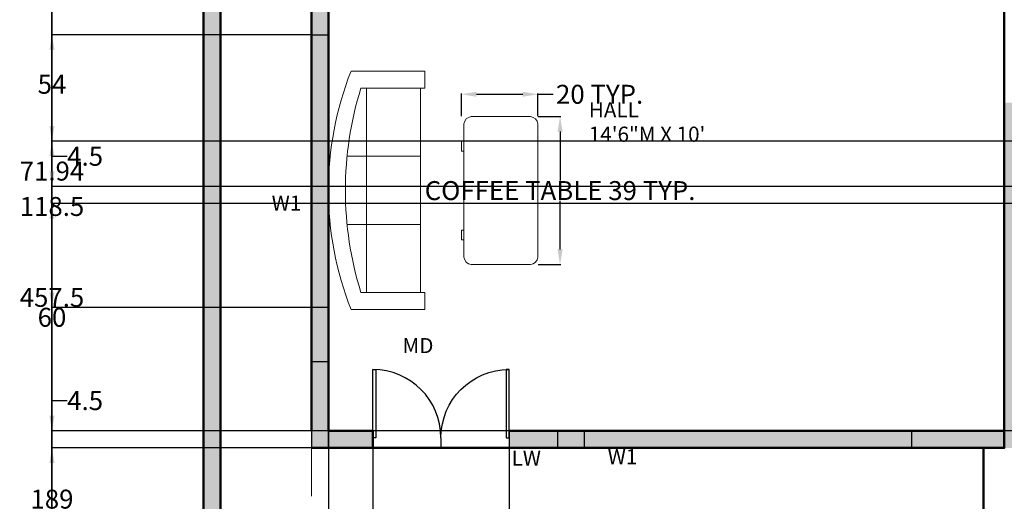
# Model space of a CAD drawing. Units: inches. Extents: x -12 to 887, y 330 to 874.
# Tile 2 of 9: x -7 to 253, y 548 to 675. Entities that reach past the tile are written whole.
import ezdxf

# ---------------------------------------------------------------- set-up
doc = ezdxf.new("R2010")
doc.units = ezdxf.units.IN
doc.header["$MEASUREMENT"] = 0
doc.linetypes.add('DASHED', pattern=[19.05, 12.7, -6.35])
for name, color, linetype, lineweight in [('A-ANNO-DIMS', 2, 'Continuous', 18), ('A-ANNO-TEXT', 3, 'Continuous', 18), ('A-AREA-IDEN', 7, 'Continuous', 18), ('A-DOOR', 4, 'Continuous', 25), ('A-FURN', 9, 'Continuous', 18), ('A-GLAZ', 4, 'Continuous', 25), ('A-WALL', 7, 'Continuous', 50), ('A-WALL-OVHD', 8, 'DASHED', 18), ('A-WALL-PATT', 5, 'Continuous', 13)]:
    doc.layers.add(name, color=color, linetype=linetype, lineweight=lineweight)
doc.styles.get("Standard").update_dxf_attribs({"font": 'arial.ttf'})
doc.dimstyles.get("Standard").update_dxf_attribs({"dimtxt": 5, "dimasz": 4, "dimexe": 0.18, "dimexo": 0.0625, "dimgap": 0.09, "dimtad": 0, "dimtih": 1, "dimtoh": 1, "dimdec": 1, "dimzin": 0, "dimdsep": 46, "dimlunit": 4, "dimtxsty": 'Standard', "dimcen": 0.09, "dimadec": 0, "dimazin": 0, "dimtfac": 1, "dimtdec": 1, "dimtofl": 0, "dimtmove": 0, "dimatfit": 3, "dimfxl": 1, "dimtolj": 1, "dimtzin": 0, "dimarcsym": 0})

# ---------------------------------------------------------------- blocks, each defined once
blk = doc.blocks.new('*U5')
for p, q in [((0, 0), (0, -6)), ((40, 0), (40, -6))]:
    blk.add_line(p, q)
blk.add_lwpolyline([(0, 0), (0, 40), (1.75, 40), (1.75, 0)], close=True)
blk.add_arc((0, 0), 40, 0, 90)
blk = doc.blocks.new('Sofa - Roundback 7 ft.')
for p, q in [((-12.00002, -32.4421), (-12.00003, -6.5971)), ((11.99997, -32.4421), (11.99998, -6.5971)), ((-36.000027, -34), (-36.000027, -11.4696)), ((-35.999844, -13.3819), (35.9998, -13.3819)), ((35.99998, -34), (35.99998, -11.4696)), ((-36.000027, -32.4421), (35.99998, -32.4421))]:
    blk.add_line(p, q)
for points in [[(-36.000027, -34), (-42.000027, -34), (-42.000027, -8)], [(41.99998, -8), (41.99998, -34), (35.99998, -34)]]:
    blk.add_lwpolyline(points)
for centre, radius, start, end in [((0, -114.25), 114.25, 68.43141, 111.5686), ((-0.00001, -127.1968), 121.1968, 72.72033, 107.2797)]:
    blk.add_arc(centre, radius, start, end)
blk = doc.blocks.new('Desk - 30 x 60 in.')
for p, q in [((-26.999995, 0), (26.999995, 0)), ((-29.999995, -27), (-29.999995, -3)), ((29.999995, -3), (29.999995, -27)), ((26.999995, -30), (-26.999995, -30)), ((-20.000005, -30), (-20.000005, -31)), ((-20.000005, -31), (-16.000005, -31)), ((-16.000005, -31), (-16.000005, -30)), ((15.999995, -31), (15.999995, -30)), ((19.999995, -31), (15.999995, -31)), ((19.999995, -30), (19.999995, -31))]:
    blk.add_line(p, q)
for centre, start, end in [((-26.499995, -3.5), 98.1301, 171.8699), ((26.499995, -3.5), 8.130102, 81.8699), ((-26.499995, -26.5), 188.1301, 261.8699), ((26.499995, -26.5), 278.1301, 351.8699)]:
    blk.add_arc(centre, 3.535534, start, end)
blk = doc.blocks.new('*D34')
at = {"layer": 'A-ANNO-DIMS', "color": 0, "lineweight": -2, "transparency": 16777216}
for p, q in [((130.31, 649.66), (136.29, 649.66)), ((136.11, 645.66), (136.11, 632.78)), ((136.11, 614.55), (136.11, 627.42)), ((130.31, 610.55), (136.29, 610.55))]:
    blk.add_line(p, q, dxfattribs=at)
at = {"layer": 'A-ANNO-DIMS', "color": 0, "transparency": 16777216}
for points in [[(135.45, 645.66), (136.78, 645.66), (136.11, 649.66)], [(135.45, 614.55), (136.78, 614.55), (136.11, 610.55)]]:
    blk.add_solid(points, dxfattribs=at)
at = {"layer": 'Defpoints', "color": 0, "transparency": 16777216}
for p in [(130.25, 649.66), (130.25, 610.55), (136.11, 610.55)]:
    blk.add_point(p, dxfattribs=at)
at = {"layer": 'A-ANNO-DIMS', "color": 0, "transparency": 16777216, "insert": (136.11, 630.1), "char_height": 5, "attachment_point": 5}
blk.add_mtext('\\A1;COFFEE TABLE 39 TYP.', dxfattribs=at)
blk = doc.blocks.new('*D35')
at = {"layer": 'A-ANNO-DIMS', "color": 0, "lineweight": -2, "transparency": 16777216}
for p, q in [((110.04, 649.72), (110.04, 655.7)), ((114.04, 655.52), (126.25, 655.52)), ((130.25, 649.72), (130.25, 655.7)), ((130.25, 655.52), (134.25, 655.52))]:
    blk.add_line(p, q, dxfattribs=at)
at = {"layer": 'A-ANNO-DIMS', "color": 0, "transparency": 16777216}
for points in [[(114.04, 656.19), (114.04, 654.86), (110.04, 655.52)], [(126.25, 656.19), (126.25, 654.86), (130.25, 655.52)]]:
    blk.add_solid(points, dxfattribs=at)
at = {"layer": 'Defpoints', "color": 0, "transparency": 16777216}
for p in [(130.25, 655.52), (110.04, 649.66), (130.25, 649.66)]:
    blk.add_point(p, dxfattribs=at)
at = {"layer": 'A-ANNO-DIMS', "color": 0, "transparency": 16777216, "insert": (146.55, 655.52), "char_height": 5, "attachment_point": 5}
blk.add_mtext('\\A1;20 TYP.', dxfattribs=at)
blk = doc.blocks.new('*D53')
at = {"layer": 'A-ANNO-DIMS', "color": 0, "lineweight": -2, "transparency": 16777216}
for p, q in [((41.86, 830.66), (1.75, 830.66)), ((1.93, 826.66), (1.93, 604.54)), ((1.93, 377.16), (1.93, 599.28)), ((41.86, 373.16), (1.75, 373.16))]:
    blk.add_line(p, q, dxfattribs=at)
at = {"layer": 'A-ANNO-DIMS', "color": 0, "transparency": 16777216}
for points in [[(1.26, 826.66), (2.59, 826.66), (1.93, 830.66)], [(1.26, 377.16), (2.59, 377.16), (1.93, 373.16)]]:
    blk.add_solid(points, dxfattribs=at)
at = {"layer": 'Defpoints', "color": 0, "transparency": 16777216}
for p in [(1.93, 830.66), (41.93, 830.66), (41.93, 373.16)]:
    blk.add_point(p, dxfattribs=at)
at = {"layer": 'A-ANNO-DIMS', "color": 0, "transparency": 16777216, "insert": (1.93, 601.91), "char_height": 5, "attachment_point": 5}
blk.add_mtext('\\A1;457.5', dxfattribs=at)
blk = doc.blocks.new('*D55')
at = {"layer": 'A-ANNO-DIMS', "color": 0, "lineweight": -2, "transparency": 16777216}
for p, q in [((70.36, 562.16), (1.75, 562.16)), ((1.93, 558.16), (1.93, 474.8)), ((1.93, 386.16), (1.93, 469.52)), ((70.36, 382.16), (1.75, 382.16))]:
    blk.add_line(p, q, dxfattribs=at)
at = {"layer": 'A-ANNO-DIMS', "color": 0, "transparency": 16777216}
for points in [[(1.26, 558.16), (2.59, 558.16), (1.93, 562.16)], [(1.26, 386.16), (2.59, 386.16), (1.93, 382.16)]]:
    blk.add_solid(points, dxfattribs=at)
at = {"layer": 'Defpoints', "color": 0, "transparency": 16777216}
for p in [(1.93, 562.16), (70.43, 562.16), (70.43, 382.16)]:
    blk.add_point(p, dxfattribs=at)
at = {"layer": 'A-ANNO-DIMS', "color": 0, "transparency": 16777216, "insert": (1.93, 472.16), "char_height": 5, "attachment_point": 5}
blk.add_mtext('\\A1;180', dxfattribs=at)
blk = doc.blocks.new('*D56')
at = {"layer": 'A-ANNO-DIMS', "color": 0, "lineweight": -2, "transparency": 16777216}
for p, q in [((1.93, 570.66), (1.93, 574.66)), ((1.93, 574.66), (5.93, 574.66)), ((74.86, 566.66), (1.75, 566.66)), ((70.36, 562.16), (1.75, 562.16)), ((1.93, 558.16), (1.93, 554.16))]:
    blk.add_line(p, q, dxfattribs=at)
at = {"layer": 'A-ANNO-DIMS', "color": 0, "transparency": 16777216}
for points in [[(1.26, 570.66), (2.59, 570.66), (1.93, 566.66)], [(1.26, 558.16), (2.59, 558.16), (1.93, 562.16)]]:
    blk.add_solid(points, dxfattribs=at)
at = {"layer": 'Defpoints', "color": 0, "transparency": 16777216}
for p in [(1.93, 566.66), (74.93, 566.66), (70.43, 562.16)]:
    blk.add_point(p, dxfattribs=at)
at = {"layer": 'A-ANNO-DIMS', "color": 0, "transparency": 16777216, "insert": (10.69, 574.66), "char_height": 5, "attachment_point": 5}
blk.add_mtext('\\A1;4.5', dxfattribs=at)
blk = doc.blocks.new('*D57')
at = {"layer": 'A-ANNO-DIMS', "color": 0, "lineweight": -2, "transparency": 16777216}
for p, q in [((74.86, 685.16), (1.75, 685.16)), ((1.93, 681.16), (1.93, 628.55)), ((1.93, 570.66), (1.93, 623.27)), ((74.86, 566.66), (1.75, 566.66))]:
    blk.add_line(p, q, dxfattribs=at)
at = {"layer": 'A-ANNO-DIMS', "color": 0, "transparency": 16777216}
for points in [[(1.26, 681.16), (2.59, 681.16), (1.93, 685.16)], [(1.26, 570.66), (2.59, 570.66), (1.93, 566.66)]]:
    blk.add_solid(points, dxfattribs=at)
at = {"layer": 'Defpoints', "color": 0, "transparency": 16777216}
for p in [(1.93, 685.16), (74.93, 685.16), (74.93, 566.66)]:
    blk.add_point(p, dxfattribs=at)
at = {"layer": 'A-ANNO-DIMS', "color": 0, "transparency": 16777216, "insert": (1.93, 625.91), "char_height": 5, "attachment_point": 5}
blk.add_mtext('\\A1;118.5', dxfattribs=at)
blk = doc.blocks.new('*D67')
at = {"layer": 'A-ANNO-DIMS', "color": 0, "lineweight": -2, "transparency": 16777216}
for p, q in [((319.86, 626.66), (1.75, 626.66)), ((1.93, 622.66), (1.93, 599.3)), ((1.93, 570.66), (1.93, 594.02)), ((319.86, 566.66), (1.75, 566.66))]:
    blk.add_line(p, q, dxfattribs=at)
at = {"layer": 'A-ANNO-DIMS', "color": 0, "transparency": 16777216}
for points in [[(1.26, 622.66), (2.59, 622.66), (1.93, 626.66)], [(1.26, 570.66), (2.59, 570.66), (1.93, 566.66)]]:
    blk.add_solid(points, dxfattribs=at)
at = {"layer": 'Defpoints', "color": 0, "transparency": 16777216}
for p in [(1.93, 626.66), (319.93, 626.66), (319.93, 566.66)]:
    blk.add_point(p, dxfattribs=at)
at = {"layer": 'A-ANNO-DIMS', "color": 0, "transparency": 16777216, "insert": (1.93, 596.66), "char_height": 5, "attachment_point": 5}
blk.add_mtext('\\A1;60', dxfattribs=at)
blk = doc.blocks.new('*D68')
at = {"layer": 'A-ANNO-DIMS', "color": 0, "lineweight": -2, "transparency": 16777216}
for p, q in [((1.93, 635.16), (1.93, 639.16)), ((1.93, 639.16), (5.93, 639.16)), ((319.86, 631.16), (1.75, 631.16)), ((319.86, 626.66), (1.75, 626.66)), ((1.93, 622.66), (1.93, 618.66))]:
    blk.add_line(p, q, dxfattribs=at)
at = {"layer": 'A-ANNO-DIMS', "color": 0, "transparency": 16777216}
for points in [[(1.26, 635.16), (2.59, 635.16), (1.93, 631.16)], [(1.26, 622.66), (2.59, 622.66), (1.93, 626.66)]]:
    blk.add_solid(points, dxfattribs=at)
at = {"layer": 'Defpoints', "color": 0, "transparency": 16777216}
for p in [(1.93, 631.16), (319.93, 631.16), (319.93, 626.66)]:
    blk.add_point(p, dxfattribs=at)
at = {"layer": 'A-ANNO-DIMS', "color": 0, "transparency": 16777216, "insert": (10.69, 639.16), "char_height": 5, "attachment_point": 5}
blk.add_mtext('\\A1;4.5', dxfattribs=at)
blk = doc.blocks.new('*D69')
at = {"layer": 'A-ANNO-DIMS', "color": 0, "lineweight": -2, "transparency": 16777216}
for p, q in [((319.86, 685.16), (1.75, 685.16)), ((1.93, 681.16), (1.93, 660.79)), ((1.93, 635.16), (1.93, 655.53)), ((319.86, 631.16), (1.75, 631.16))]:
    blk.add_line(p, q, dxfattribs=at)
at = {"layer": 'A-ANNO-DIMS', "color": 0, "transparency": 16777216}
for points in [[(1.26, 681.16), (2.59, 681.16), (1.93, 685.16)], [(1.26, 635.16), (2.59, 635.16), (1.93, 631.16)]]:
    blk.add_solid(points, dxfattribs=at)
at = {"layer": 'Defpoints', "color": 0, "transparency": 16777216}
for p in [(1.93, 685.16), (319.93, 685.16), (319.93, 631.16)]:
    blk.add_point(p, dxfattribs=at)
at = {"layer": 'A-ANNO-DIMS', "color": 0, "transparency": 16777216, "insert": (1.93, 658.16), "char_height": 5, "attachment_point": 5}
blk.add_mtext('\\A1;54', dxfattribs=at)
blk = doc.blocks.new('*D76')
at = {"layer": 'A-ANNO-DIMS', "color": 0, "lineweight": -2, "transparency": 16777216}
for p, q in [((74.93, 566.6), (74.93, 332.98)), ((86.65, 566.6), (86.65, 332.98)), ((78.93, 333.16), (82.65, 333.16)), ((86.65, 333.16), (90.65, 333.16))]:
    blk.add_line(p, q, dxfattribs=at)
at = {"layer": 'A-ANNO-DIMS', "color": 0, "transparency": 16777216}
for points in [[(78.93, 333.83), (78.93, 332.49), (74.93, 333.16)], [(82.65, 333.83), (82.65, 332.49), (86.65, 333.16)]]:
    blk.add_solid(points, dxfattribs=at)
at = {"layer": 'Defpoints', "color": 0, "transparency": 16777216}
for p in [(74.93, 566.66), (86.65, 566.66), (86.65, 333.16)]:
    blk.add_point(p, dxfattribs=at)
at = {"layer": 'A-ANNO-DIMS', "color": 0, "transparency": 16777216, "insert": (98.91, 333.16), "char_height": 5, "attachment_point": 5}
blk.add_mtext('\\A1;11.72', dxfattribs=at)
blk = doc.blocks.new('*D77')
at = {"layer": 'A-ANNO-DIMS', "color": 0, "lineweight": -2, "transparency": 16777216}
for p, q in [((86.65, 566.6), (86.65, 332.98)), ((122.7, 566.6), (122.7, 332.98)), ((90.65, 333.16), (96.13, 333.16)), ((118.7, 333.16), (113.22, 333.16))]:
    blk.add_line(p, q, dxfattribs=at)
at = {"layer": 'A-ANNO-DIMS', "color": 0, "transparency": 16777216}
for points in [[(90.65, 333.83), (90.65, 332.49), (86.65, 333.16)], [(118.7, 333.83), (118.7, 332.49), (122.7, 333.16)]]:
    blk.add_solid(points, dxfattribs=at)
at = {"layer": 'Defpoints', "color": 0, "transparency": 16777216}
for p in [(86.65, 566.66), (122.7, 566.66), (122.7, 333.16)]:
    blk.add_point(p, dxfattribs=at)
at = {"layer": 'A-ANNO-DIMS', "color": 0, "transparency": 16777216, "insert": (104.67, 333.16), "char_height": 5, "attachment_point": 5}
blk.add_mtext('\\A1;36.05', dxfattribs=at)
blk = doc.blocks.new('*D82')
at = {"layer": 'A-ANNO-DIMS', "color": 0, "lineweight": -2, "transparency": 16777216}
for p, q in [((70.36, 671.22), (1.75, 671.22)), ((1.93, 667.22), (1.93, 637.89)), ((1.93, 603.27), (1.93, 632.6)), ((70.36, 599.27), (1.75, 599.27))]:
    blk.add_line(p, q, dxfattribs=at)
at = {"layer": 'A-ANNO-DIMS', "color": 0, "transparency": 16777216}
for points in [[(1.26, 667.22), (2.59, 667.22), (1.93, 671.22)], [(1.26, 603.27), (2.59, 603.27), (1.93, 599.27)]]:
    blk.add_solid(points, dxfattribs=at)
at = {"layer": 'Defpoints', "color": 0, "transparency": 16777216}
for p in [(70.43, 671.22), (1.93, 599.27), (70.43, 599.27)]:
    blk.add_point(p, dxfattribs=at)
at = {"layer": 'A-ANNO-DIMS', "color": 0, "transparency": 16777216, "insert": (1.93, 635.24), "char_height": 5, "attachment_point": 5}
blk.add_mtext('\\A1;71.94', dxfattribs=at)
blk = doc.blocks.new('*D101')
at = {"layer": 'A-ANNO-DIMS', "color": 0, "lineweight": -2, "transparency": 16777216}
for p, q in [((493.01, 643.16), (1.75, 643.16)), ((1.93, 639.16), (1.93, 551.3)), ((1.93, 458.16), (1.93, 546.02)), ((493.01, 454.16), (1.75, 454.16))]:
    blk.add_line(p, q, dxfattribs=at)
at = {"layer": 'A-ANNO-DIMS', "color": 0, "transparency": 16777216}
for points in [[(1.26, 639.16), (2.59, 639.16), (1.93, 643.16)], [(1.26, 458.16), (2.59, 458.16), (1.93, 454.16)]]:
    blk.add_solid(points, dxfattribs=at)
at = {"layer": 'Defpoints', "color": 0, "transparency": 16777216}
for p in [(1.93, 643.16), (493.07, 643.16), (493.07, 454.16)]:
    blk.add_point(p, dxfattribs=at)
at = {"layer": 'A-ANNO-DIMS', "color": 0, "transparency": 16777216, "insert": (1.93, 548.66), "char_height": 5, "attachment_point": 5}
blk.add_mtext('\\A1;189', dxfattribs=at)
blk = doc.blocks.new('*D102')
at = {"layer": 'A-ANNO-DIMS', "color": 0, "lineweight": -2, "transparency": 16777216}
for p, q in [((493.01, 821.66), (1.75, 821.66)), ((1.93, 817.66), (1.93, 735.05)), ((1.93, 647.16), (1.93, 729.77)), ((493.01, 643.16), (1.75, 643.16))]:
    blk.add_line(p, q, dxfattribs=at)
at = {"layer": 'A-ANNO-DIMS', "color": 0, "transparency": 16777216}
for points in [[(1.26, 817.66), (2.59, 817.66), (1.93, 821.66)], [(1.26, 647.16), (2.59, 647.16), (1.93, 643.16)]]:
    blk.add_solid(points, dxfattribs=at)
at = {"layer": 'Defpoints', "color": 0, "transparency": 16777216}
for p in [(1.93, 821.66), (493.07, 821.66), (493.07, 643.16)]:
    blk.add_point(p, dxfattribs=at)
at = {"layer": 'A-ANNO-DIMS', "color": 0, "transparency": 16777216, "insert": (1.93, 732.41), "char_height": 5, "attachment_point": 5}
blk.add_mtext('\\A1;178.5', dxfattribs=at)

msp = doc.modelspace()

# ---------------------------------------------------------------- hatches: boundary and pattern name
at = {"layer": 'A-WALL-PATT'}
h = msp.add_hatch(color=256, dxfattribs=at)
h.dxf.hatch_style = 1
h.paths.add_polyline_path([(253.4263, 830.6611), (94.575, 830.6611), (94.575, 821.6611), (198.9263, 821.6611), (198.9263, 783.3094), (203.4263, 783.3094), (203.4263, 821.6611), (253.4263, 821.6611)], flags=17)
h.paths.add_polyline_path([(415.4263, 830.6611), (392.9263, 830.6611), (392.9263, 821.6611), (410.9263, 821.6611), (410.9263, 701.6611), (410.9263, 382.1611), (392.9263, 382.1611), (392.9263, 450.1611), (383.9263, 450.1611), (383.9263, 382.1611), (253.4263, 382.1611), (46.4263, 382.1611), (46.4263, 821.6611), (67.3199, 821.6611), (67.3199, 830.6611), (41.9263, 830.6611), (41.9263, 373.1611), (253.4263, 373.1611), (415.4263, 373.1611)])
h.paths.add_polyline_path([(364.023, 830.6611), (288.8031, 830.6611), (288.8031, 821.6611), (364.023, 821.6611)], flags=17)
h.paths.add_polyline_path([(257.9263, 821.6611), (253.4263, 821.6611), (253.4263, 749.6611), (203.4263, 749.6611), (203.4263, 759.3094), (198.9263, 759.3094), (198.9263, 745.1611), (253.4263, 745.1611), (253.4263, 735.8547), (257.9263, 735.8547)], flags=17)
h.paths.add_polyline_path([(257.9263, 653.338), (257.0311, 653.338), (253.4263, 653.338), (253.4263, 579.1607), (257.9263, 579.1607)], flags=17)
h.paths.add_polyline_path([(323.9263, 685.1611), (328.2749, 685.1611), (328.2749, 689.6611), (257.9263, 689.6611), (257.9263, 685.1611), (319.9263, 685.1611), (319.9263, 631.1611), (257.9263, 631.1611), (257.9263, 626.6611), (319.9263, 626.6611), (319.9263, 566.6611), (286.6409, 566.6611, -0.00931598), (286.6576, 565.7658), (286.6576, 562.1611), (383.9263, 562.1611), (383.9263, 566.6611), (323.9263, 566.6611)], flags=17)
h.paths.add_polyline_path([(142.5107, 566.6611), (135.5357, 566.6611), (135.5357, 562.1611), (142.5107, 562.1611)], flags=17)
h.paths.add_polyline_path([(253.4263, 566.6611), (229.0035, 566.6611), (229.0035, 562.1611), (253.4263, 562.1611)], flags=17)
h.paths.add_polyline_path([(262.6261, 566.6611), (257.9263, 566.6611), (257.9263, 562.1611), (262.6261, 562.1611)], flags=17)
h.paths.add_polyline_path([(392.9263, 553.5254), (383.9263, 553.5254), (383.9263, 454.1611), (392.9263, 454.1611)], flags=17)
h.paths.add_polyline_path([(353.8031, 418.1611), (247.9263, 418.1611), (247.9263, 414.1611), (353.8031, 414.1611)], flags=17)
h.paths.add_polyline_path([(374.959, 454.1611), (272.0195, 454.1611), (272.0195, 450.1611), (374.959, 450.1611)], flags=17)
h.paths.add_polyline_path([(254.2006, 454.1611), (247.9263, 454.1611), (247.9263, 450.1611), (254.2006, 450.1611)], flags=17)
h = msp.add_hatch(color=256, dxfattribs=at)
h.dxf.hatch_style = 1
h.paths.add_polyline_path([(94.575, 830.6611), (67.3199, 830.6611), (67.3199, 821.6611), (70.4263, 821.6611), (79.4263, 821.6611), (94.575, 821.6611)])
h.paths.add_polyline_path([(288.8031, 830.6611), (257.9263, 830.6611), (253.4263, 830.6611), (253.4263, 821.6611), (288.8031, 821.6611)])
h.paths.add_polyline_path([(74.9263, 696.9265), (70.4263, 696.9265), (70.4263, 678.4656), (74.9263, 678.4656)])
h.paths.add_polyline_path([(74.9263, 584.8756), (70.4263, 584.8756), (70.4263, 562.1611), (74.9263, 562.1611)])
h.paths.add_polyline_path([(135.5357, 566.6611), (122.6994, 566.6611), (122.6994, 562.1611), (135.5357, 562.1611)])
h.paths.add_polyline_path([(257.9263, 579.1607), (253.4263, 579.1607), (253.4263, 562.1611), (257.9263, 562.1611)])
h.paths.add_polyline_path([(272.0195, 454.1611), (254.2006, 454.1611), (254.2006, 450.1611), (272.0195, 450.1611)])
h.paths.add_polyline_path([(392.9263, 454.1611), (374.959, 454.1611), (374.959, 450.1611), (383.9263, 450.1611), (392.9263, 450.1611)])
h.paths.add_polyline_path([(493.0683, 466.4171), (488.5683, 466.4171), (488.5683, 450.1611), (493.0683, 450.1611)])
h.paths.add_polyline_path([(568.6302, 454.1611), (555.938, 454.1611), (555.938, 450.1611), (568.6302, 450.1611)])
h.paths.add_polyline_path([(493.0683, 594.9471), (488.5683, 594.9471), (488.5683, 569.5862), (493.0683, 569.5862)])
h.paths.add_polyline_path([(690.1615, 454.1611), (672.3426, 454.1611), (672.3426, 450.1611), (690.1615, 450.1611)])
h.paths.add_polyline_path([(811.0683, 454.1611), (793.101, 454.1611), (793.101, 450.1611), (802.0683, 450.1611), (811.0683, 450.1611)])
h.paths.add_polyline_path([(811.0683, 578.3606), (802.0683, 578.3606), (802.0683, 566.6611), (802.0683, 553.5254), (811.0683, 553.5254)])
h.paths.add_polyline_path([(811.0683, 701.6611), (802.0683, 701.6611), (802.0683, 689.9616), (802.0683, 676.8259), (811.0683, 676.8259)])
h.paths.add_polyline_path([(811.0683, 830.6611), (782.165, 830.6611), (782.165, 821.6611), (802.0683, 821.6611), (811.0683, 821.6611)])
h.paths.add_polyline_path([(706.9451, 830.6611), (671.5683, 830.6611), (671.5683, 821.6611), (706.9451, 821.6611)])
h.paths.add_polyline_path([(512.717, 830.6611), (485.4619, 830.6611), (485.4619, 821.6611), (488.5683, 821.6611), (512.717, 821.6611)])
h.paths.add_polyline_path([(392.9263, 697.8668), (383.9263, 697.8668), (383.9263, 689.6611), (383.9263, 676.5034), (392.9263, 676.5034)])
h.paths.add_polyline_path([(392.9263, 830.6611), (364.023, 830.6611), (364.023, 821.7357), (392.9263, 821.7357)])
h.paths.add_polyline_path([(392.9263, 619.0434), (383.9263, 619.0434), (383.9263, 588.7499), (392.9263, 588.7499)])
h.paths.add_polyline_path([(392.9263, 578.3606), (383.9263, 578.3606), (383.9263, 566.6611), (383.9263, 553.5254), (392.9263, 553.5254)])
h.paths.add_polyline_path([(257.9263, 699.8547), (253.4263, 699.8547), (253.4263, 697.1611), (253.4263, 677.338), (257.9263, 677.338)])
h.paths.add_polyline_path([(493.0683, 714.3785), (488.5683, 714.3785), (488.5683, 689.6611), (493.0683, 689.6611)])
h.paths.add_polyline_path([(74.9263, 491.4191), (70.4263, 491.4191), (70.4263, 480.7097), (74.9263, 480.7097)])
h = msp.add_hatch(color=256, dxfattribs=at)
h.dxf.hatch_style = 1
h.paths.add_polyline_path([(86.6469, 566.6611), (74.9263, 566.6611), (74.9263, 562.1611), (86.6469, 562.1611)])
h.paths.add_polyline_path([(74.9263, 599.271), (70.4263, 599.271), (70.4263, 584.8756), (74.9263, 584.8756)])
h.paths.add_polyline_path([(74.9263, 678.4656), (70.4263, 678.4656), (70.4263, 671.2153), (74.9263, 671.2153)])
h.paths.add_polyline_path([(74.9263, 709.2627), (70.4263, 709.2627), (70.4263, 696.9265), (74.9263, 696.9265)])
h.paths.add_polyline_path([(74.9263, 821.6611), (70.4263, 821.6611), (70.4263, 749.8953), (74.9263, 749.8953)])
h.paths.add_polyline_path([(383.9263, 689.6611), (352.3064, 689.6611), (352.3064, 686.0564, -0.00931598), (352.2897, 685.1611), (383.9263, 685.1611)])
h.paths.add_polyline_path([(392.9263, 706.6608), (383.9263, 706.6608), (383.9263, 701.6611), (383.9263, 697.8668), (392.9263, 697.8668)])
h.paths.add_polyline_path([(392.9263, 821.7357), (383.9263, 821.7357), (383.9263, 751.0224), (383.9263, 742.7561), (392.9263, 742.7561)])
h.paths.add_polyline_path([(392.9263, 676.5034), (383.9263, 676.5034), (383.9263, 619.0434), (392.9263, 619.0434)])
h.paths.add_polyline_path([(392.9263, 588.7499), (383.9263, 588.7499), (383.9263, 578.3606), (392.9263, 578.3606)])
h = msp.add_hatch(color=256, dxfattribs=at)
h.dxf.hatch_style = 1
h.paths.add_polyline_path([(74.9263, 749.8953), (70.4263, 749.8953), (70.4263, 709.2627), (74.9263, 709.2627)])
h.paths.add_polyline_path([(74.9263, 671.2153), (70.4263, 671.2153), (70.4263, 599.271), (74.9263, 599.271)])
h.paths.add_polyline_path([(229.0035, 566.6611), (142.5107, 566.6611), (142.5107, 562.1611), (229.0035, 562.1611)])
h.paths.add_polyline_path([(392.9263, 742.7561), (383.9263, 742.7561), (383.9263, 706.6608), (392.9263, 706.6608)])
h.paths.add_polyline_path([(656.7304, 454.1611), (582.6585, 454.1611), (582.6585, 450.1611), (656.7304, 450.1611)])
h.paths.add_polyline_path([(493.0683, 557.2595), (488.5683, 557.2595), (488.5683, 492.3446), (493.0683, 492.3446)])
h.paths.add_polyline_path([(493.0683, 781.3634), (488.5683, 781.3634), (488.5683, 728.8273), (493.0683, 728.8273)])
h.paths.add_polyline_path([(811.0683, 756.0738), (802.0683, 756.0738), (802.0683, 707.8935), (811.0683, 707.8935)])

# ---------------------------------------------------------------- linework, layer by layer
at = {"layer": 'A-GLAZ'}
for points in [[(70.4263, 671.2153), (74.9263, 671.2153), (74.9263, 599.271), (70.4263, 599.271)], [(122.6994, 562.1611), (135.5357, 562.1611), (135.5357, 566.6611), (122.6994, 566.6611)], [(142.5107, 562.1611), (229.0035, 562.1611), (229.0035, 566.6611), (142.5107, 566.6611)]]:
    msp.add_lwpolyline(points, close=True, dxfattribs=at)
msp.add_lwpolyline([(70.4263, 562.1611), (74.9263, 562.1611), (74.9263, 584.8756), (70.4263, 584.8756), (70.4263, 562.1611)], dxfattribs=at)
at = {"layer": 'A-WALL'}
for p, q in [((70.4263, 821.6611), (70.4263, 566.6611)), ((122.6994, 566.6611), (253.4263, 566.6611)), ((70.4263, 562.1611), (122.6994, 562.1611)), ((247.9263, 562.1611), (247.9263, 454.1611))]:
    msp.add_line(p, q, dxfattribs=at)
msp.add_lwpolyline([(41.9263, 830.6611), (253.4263, 830.6611), (257.9263, 830.6611), (415.4263, 830.6611), (415.4263, 373.1611), (253.4263, 373.1611), (41.9263, 373.1611)], close=True, dxfattribs=at)
for points in [[(247.9263, 450.1611), (383.9263, 450.1611), (383.9263, 382.1611), (253.4263, 382.1611), (46.4263, 382.1611), (46.4263, 821.6611), (70.4263, 821.6611), (79.4263, 821.6611), (198.9263, 821.6611), (198.9263, 745.1611)], [(86.6469, 562.1611), (86.6469, 566.6611), (74.9263, 566.6611), (74.9263, 685.1611), (198.9263, 685.1611), (198.9263, 745.1611), (253.4263, 745.1611), (253.4263, 697.1611), (253.4263, 562.1611), (122.6469, 562.1611)]]:
    msp.add_lwpolyline(points, dxfattribs=at)
at = {"layer": 'A-WALL-OVHD'}
msp.add_line((70.4263, 562.1611), (70.4263, 382.1611), dxfattribs=at)

# ---------------------------------------------------------------- block references
at = {"layer": 'A-DOOR', "yscale": 0.4502876055566471, "zscale": 0.4502876055566471}
for p, xscale in [((86.6469, 564.8628), 0.4502876055566471), ((122.6699, 564.8628), -0.4502876055566471)]:
    msp.add_blockref('*U5', p, dxfattribs=dict(at, xscale=xscale))
at = {"layer": 'A-FURN'}
for name, p, xscale, yscale, zscale, rotation in [('Sofa - Roundback 7 ft.', (74.9263, 630.1701), 0.7491386344428914, 0.7491386344428914, 0.7491386344428914, 90), ('Desk - 30 x 60 in.', (130.2469, 630.1027), 0.6517754393069863, 0.6517754393069863, 0.6517754393069863, 270)]:
    msp.add_blockref(name, p, dxfattribs=dict(at, xscale=xscale, yscale=yscale, zscale=zscale, rotation=rotation))

# ---------------------------------------------------------------- texts
at = {"layer": 'A-ANNO-TEXT'}
for s, p in [('W1', (59.9403, 624.7943)), ('MD', (94.4911, 587.188)), ('W1', (148.6933, 557.8652)), ('LW', (123.3049, 557.466))]:
    msp.add_text(s, height=4, dxfattribs=at).set_placement(p)
at = {"layer": 'A-AREA-IDEN'}
for s, p in [('HALL', (143.7042, 649.4086)), ('14\'6"M X 10\'', (143.7042, 642.983))]:
    msp.add_text(s, height=4, dxfattribs=at).set_placement(p)

# ---------------------------------------------------------------- dimensions: what is measured, and where the dimension line sits
at = {"layer": 'A-ANNO-DIMS'}
for base, p1, p2, override, picture, middle in [((1.9263, 830.6611), (41.9263, 373.1611), (41.9263, 830.6611), {"dimdec": 1, "dimlfac": 1, "dimrnd": 0, "dimzin": 0, "dimdsep": 46, "dimlunit": 2}, '*D53', (1.9263, 601.9111)), ((1.9263, 821.6611), (493.0683, 643.1611), (493.0683, 821.6611), {"dimdec": 1, "dimlfac": 1, "dimrnd": 0, "dimzin": 0, "dimdsep": 46, "dimlunit": 2}, '*D102', (1.9263, 732.4111)), ((1.9263, 685.1611), (74.9263, 566.6611), (74.9263, 685.1611), {"dimdec": 1, "dimlfac": 1, "dimrnd": 0, "dimzin": 0, "dimdsep": 46, "dimlunit": 2}, '*D57', (1.9263, 625.9111)), ((1.9263, 685.1611), (319.9263, 631.1611), (319.9263, 685.1611), {"dimdec": 0, "dimlfac": 1, "dimrnd": 0, "dimzin": 0, "dimdsep": 46, "dimlunit": 2}, '*D69', (1.9263, 658.1611)), ((1.9263, 599.271), (70.4263, 671.2153), (70.4263, 599.271), {"dimdec": 2, "dimlfac": 1, "dimrnd": 0, "dimzin": 0, "dimdsep": 46, "dimlunit": 2}, '*D82', (1.9263, 635.2432)), ((1.9263, 643.1611), (493.0683, 454.1611), (493.0683, 643.1611), {"dimdec": 0, "dimlfac": 1, "dimrnd": 0, "dimzin": 0, "dimdsep": 46, "dimlunit": 2}, '*D101', (1.9263, 548.6611)), ((1.9263, 631.1611), (319.9263, 626.6611), (319.9263, 631.1611), {"dimdec": 1, "dimlfac": 1, "dimrnd": 0, "dimzin": 0, "dimdsep": 46, "dimlunit": 2}, '*D68', (10.6872, 639.1611)), ((1.9263, 626.6611), (319.9263, 566.6611), (319.9263, 626.6611), {"dimdec": 0, "dimlfac": 1, "dimrnd": 0, "dimzin": 0, "dimdsep": 46, "dimlunit": 2}, '*D67', (1.9263, 596.6611)), ((1.9263, 566.6611), (70.4263, 562.1611), (74.9263, 566.6611), {"dimdec": 1, "dimlfac": 1, "dimrnd": 0, "dimzin": 0, "dimdsep": 46, "dimlunit": 2}, '*D56', (10.6872, 574.6611)), ((1.9263, 562.1611), (70.4263, 382.1611), (70.4263, 562.1611), {"dimdec": 0, "dimlfac": 1, "dimrnd": 0, "dimzin": 0, "dimdsep": 46, "dimlunit": 2}, '*D55', (1.9263, 472.1611))]:
    dim = msp.add_linear_dim(base=base, p1=p1, p2=p2, angle=90, dimstyle='Standard', override=override, dxfattribs=at)
    dim.commit()
    dim.dimension.update_dxf_attribs({"geometry": picture, "text_midpoint": middle})
dim = msp.add_linear_dim(base=(130.2469, 655.5219), p1=(110.0419, 649.6559), p2=(130.2469, 649.6559), text='<> TYP.', dimstyle='Standard', override={"dimdec": 0, "dimrnd": 0, "dimzin": 0, "dimlunit": 2}, dxfattribs=at)
dim.commit()
dim.dimension.update_dxf_attribs({"geometry": '*D35', "text_midpoint": (146.5487, 655.5219)})
dim = msp.add_linear_dim(base=(136.1129, 610.5494), p1=(130.2469, 649.6559), p2=(130.2469, 610.5494), angle=270, text='COFFEE TABLE <> TYP.', dimstyle='Standard', override={"dimdec": 0, "dimrnd": 0, "dimzin": 0, "dimlunit": 2}, dxfattribs=at)
dim.commit()
dim.dimension.update_dxf_attribs({"geometry": '*D34', "text_midpoint": (136.1129, 630.1027)})
for base, p1, p2, picture, middle in [((86.6469, 333.1611), (74.9263, 566.6611), (86.6469, 566.6611), '*D76', (98.9122, 333.1611)), ((122.6994, 333.1611), (86.6469, 566.6611), (122.6994, 566.6611), '*D77', (104.6732, 333.1611))]:
    dim = msp.add_linear_dim(base=base, p1=p1, p2=p2, dimstyle='Standard', override={"dimdec": 2, "dimlfac": 1, "dimrnd": 0, "dimzin": 0, "dimdsep": 46, "dimlunit": 2}, dxfattribs=at)
    dim.commit()
    dim.dimension.update_dxf_attribs({"geometry": picture, "text_midpoint": middle})

doc.saveas('drawing.dxf')
